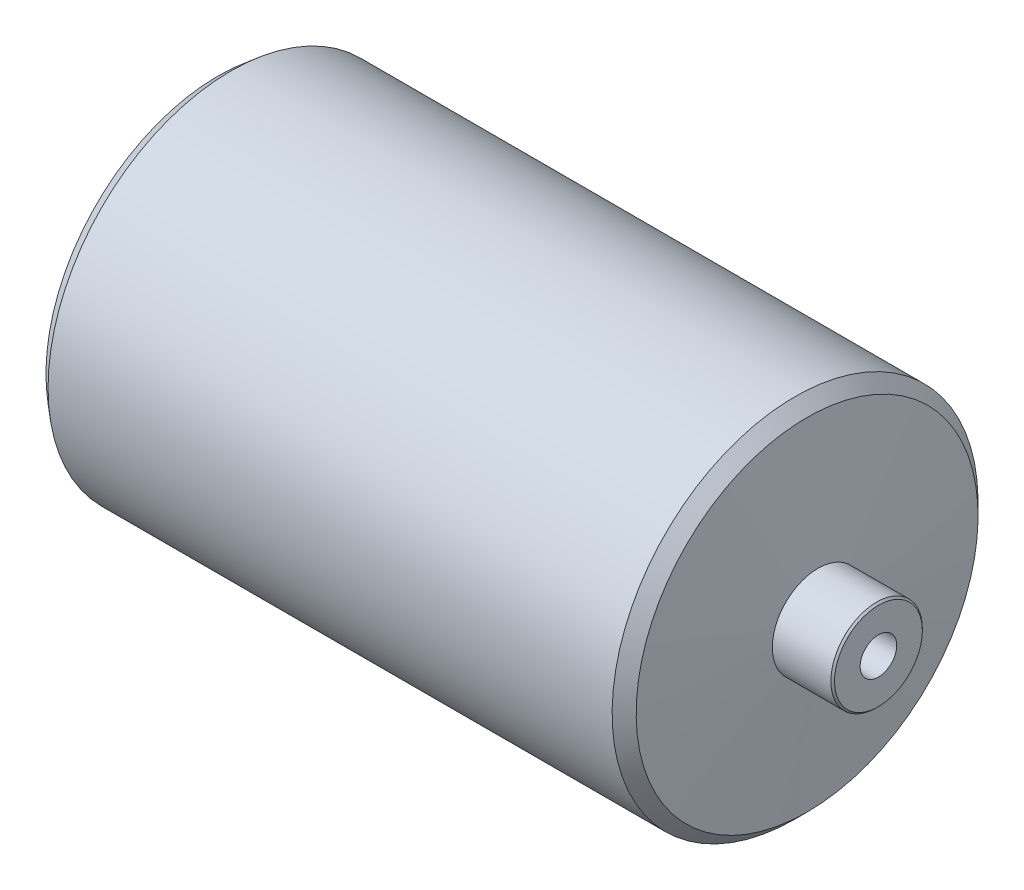
from build123d import *
from OCP.BRepFilletAPI import BRepFilletAPI_MakeChamfer

# Parameters (mm, degrees)
JOURNAL_CHAMFER_0_5MM_A_SIZE  = 0.5
JOURNAL_CHAMFER_0_5MM_B_SIZE  = 0.5
BODY_EDGE_CHAMFER_3MM_SIZE    = 3
BODY_EDGE_CHAMFER_3MM_SIZE2   = 3.300188603
CENTRE_HOLE_10X59_END_A_D     = 10
CENTRE_HOLE_10X59_END_A_DEPTH = 59
CENTRE_HOLE_10X59_END_B_D     = 10
CENTRE_HOLE_10X59_END_B_DEPTH = 59


with BuildPart() as part:
    # Roller Profile Sketch → Roller Body (revolve)
    with BuildSketch(Plane.XY):
        Polygon((0, 0), (0, 12.5), (16.5, 12.5), (19.780824882, 50), (180.219175118, 50), (183.5, 12.5), (200, 12.5), (200, 0), align=None)
    revolve(axis=Axis((200, 0, 0), (-1, 0, 0)))

    # Journal Chamfer 0.5mm A
    journal_chamfer_0_5mm_a_edges = [part.edges().sort_by_distance(p)[0] for p in [
        (200, -12.5, 0),
    ]]
    chamfer(journal_chamfer_0_5mm_a_edges, length=JOURNAL_CHAMFER_0_5MM_A_SIZE)

    # Journal Chamfer 0.5mm B
    journal_chamfer_0_5mm_b_edges = [part.edges().sort_by_distance(p)[0] for p in [
        (0, -12.5, 0),
    ]]
    chamfer(journal_chamfer_0_5mm_b_edges, length=JOURNAL_CHAMFER_0_5MM_B_SIZE)

    # Body Edge Chamfer 3mm: one chamfer whose edges measure the first distance from different faces: ONE call of the kernel's chamfer builder (chamfer() names one face for all edges)
    body_edge_chamfer_3mm_edges_1 = [part.edges().sort_by_distance(p)[0] for p in [
        (180.219175118, -50, 0),
    ]]
    body_edge_chamfer_3mm_side_1 = [part.faces().sort_by_distance(p)[0] for p in [
        (100, -50, 0),
    ]]
    body_edge_chamfer_3mm_edges_2 = [part.edges().sort_by_distance(p)[0] for p in [
        (19.780824882, -50, 0),
    ]]
    body_edge_chamfer_3mm_side_2 = [part.faces().sort_by_distance(p)[0] for p in [
        (18.140412441, -31.25, 0),
    ]]
    body_edge_chamfer_3mm = BRepFilletAPI_MakeChamfer(part.part.solid().wrapped)
    for e in body_edge_chamfer_3mm_edges_1:
        body_edge_chamfer_3mm.Add(BODY_EDGE_CHAMFER_3MM_SIZE, BODY_EDGE_CHAMFER_3MM_SIZE2, e.wrapped, body_edge_chamfer_3mm_side_1[0].wrapped)  # the first distance lies on this face
    for e in body_edge_chamfer_3mm_edges_2:
        body_edge_chamfer_3mm.Add(BODY_EDGE_CHAMFER_3MM_SIZE, BODY_EDGE_CHAMFER_3MM_SIZE2, e.wrapped, body_edge_chamfer_3mm_side_2[0].wrapped)  # the first distance lies on this face
    add(Compound.cast(body_edge_chamfer_3mm.Shape()), mode=Mode.REPLACE)

    # Centre Hole Ø10x59 End A
    with Locations(Plane(origin=(200, 0, 0), x_dir=(0, 0, -1), z_dir=(1, 0, 0))):
        with Locations((0, 0)):
            Hole(CENTRE_HOLE_10X59_END_A_D / 2, depth=CENTRE_HOLE_10X59_END_A_DEPTH)

    # Centre Hole Ø10x59 End B
    with Locations(Plane.ZY):
        with Locations((0, 0)):
            Hole(CENTRE_HOLE_10X59_END_B_D / 2, depth=CENTRE_HOLE_10X59_END_B_DEPTH)


solid = part.part
